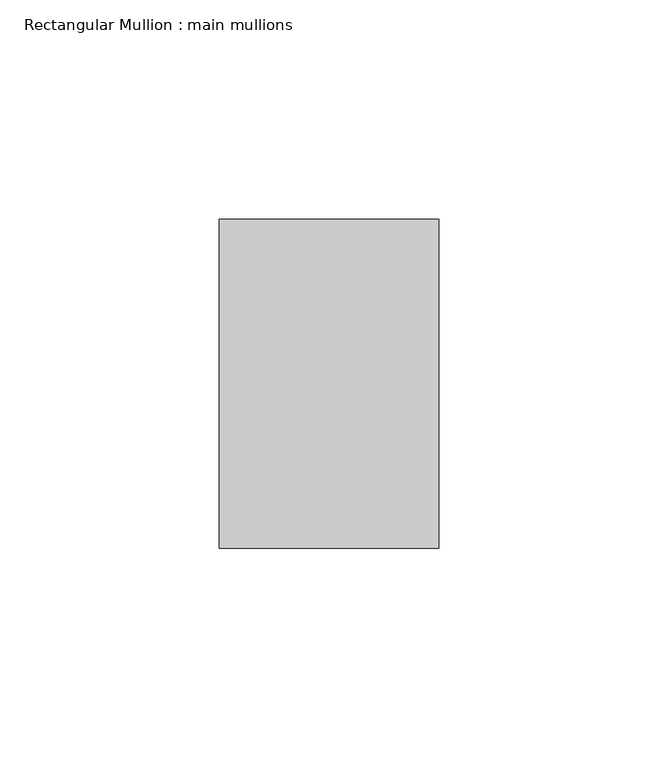
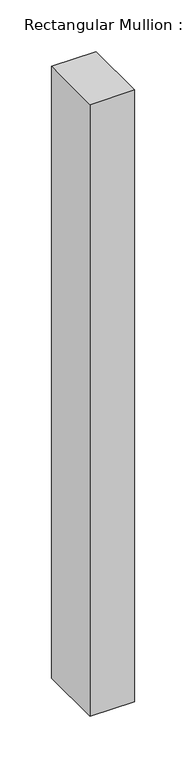
"""IFC4 building model written with IfcOpenShell, lengths in millimetres: member geometry, Rectangular Mullion : main mullions."""

from ifc_helpers import new_model, si_unit, frame, origin, place, context, project, spatial, polyline, outline, extrude, source, transform, mapped, element, save


def rectangular_mullion_main_mullions_6707c5fc(model_context):
    return source(origin(), model_context, "Body", "SweptSolid", [
        extrude(outline(polyline([(25.0, 37.5), (25.0, -37.5), (-25.0, -37.5), (-25.0, 37.5), (25.0, 37.5)])), frame((0.0, 0.0, -725.0), z_axis=(0.0, 0.0, 1.0), x_axis=(1.0, 0.0, 0.0)), (0.0, 0.0, 1.0), 725.0),
    ])


if __name__ == "__main__":
    model = new_model("IFC4")
    model_context = context("Model", 3, world=origin())
    ifc_project = project(units=[si_unit("LENGTHUNIT", "METRE", prefix="MILLI")], contexts=[model_context])
    site = spatial("IfcSite", under=ifc_project)
    building = spatial("IfcBuilding", under=site)
    placement = place(None, origin())
    rectangular_mullion_main_mullions_shape = rectangular_mullion_main_mullions_6707c5fc(model_context)
    element("IfcMember", 1, ObjectType="Rectangular Mullion : main mullions", at=placement, inside=building, context=model_context, shape_type="MappedRepresentation", body=[
        mapped(rectangular_mullion_main_mullions_shape, transform((0.0, 0.0, 0.0), x_axis=(1.0, 0.0, 0.0), y_axis=(0.0, 1.0, 0.0), z_axis=(0.0, 0.0, 1.0))),
    ])
    save(model, "model.ifc")

# Revit data of these elements
# Type "Rectangular Mullion : main mullions"
#   built-in parameter 1007304 = 0.246063 (stored number, unit not read)
#   built-in parameter 1007301 = 0.082021 (stored number, unit not read)
#   built-in parameter 1007300 = 0.082021 (stored number, unit not read)
# Element 1 (IfcMember, "Rectangular Mullion : main mullions")
#   Materials on its faces: "Aluminum"
# Materials
#   "Aluminum": class "Metal", colour RGB 136 136 136, transparency 0, Description = "Aluminum 6061", Cost = 0
